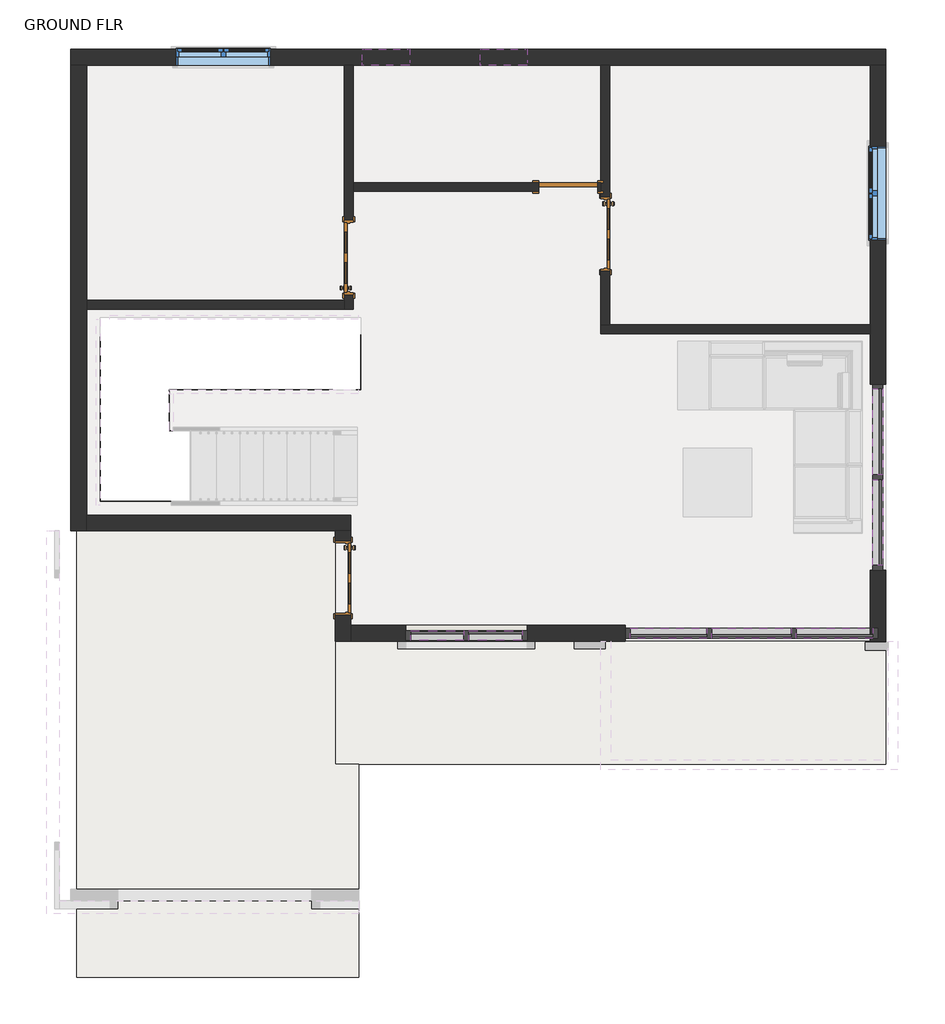
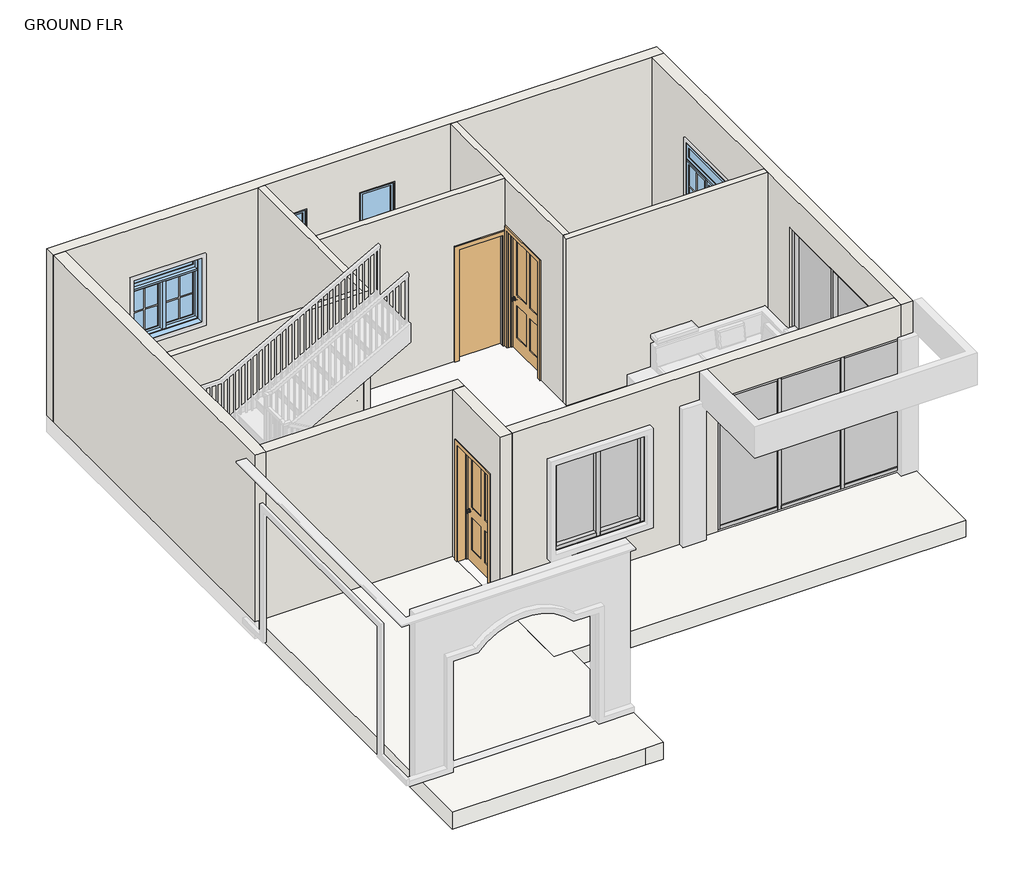
# One storey, part 1 of 3: 24 members, 11 walls, 7 plates, 7 slabs, 4 doors, 4 windows.
"""IFC4 building model written with IfcOpenShell, lengths in millimetres."""

from ifc_helpers import new_model, si_unit, frame, origin, origin_with_axes, place, context, project, spatial, polyline, outline, extrude, faceted_brep, transform, mapped, element, save
from components import door_2d5c49d3, door_c2926031, door_d8f5dbb5, member_5f1d7e17, member_aaf6ec4e, member_f0fea5a5, member_ee409385, member_a27facc5, member_7a2ba7d2, member_30308bf7, member_456a42a1, system_panel_glazed_72e6272a, system_panel_glazed_683b098e, system_panel_glazed_7ebbbc7e, system_panel_glazed_68324572, window_6846e476, window_ba962a69, window_3911def3

model = new_model("IFC4")

# Units and contexts
model_context = context("Model", 3, world=origin())
ifc_project = project(units=[si_unit("LENGTHUNIT", "METRE", prefix="MILLI")], contexts=[model_context])

# Site, building, storey
site = spatial("IfcSite", under=ifc_project)
building = spatial("IfcBuilding", under=site)
storey = spatial("IfcBuildingStorey", under=building, Name="GROUND FLR", Elevation=304.8)

# Doors
placement = place(None, origin())
door_shape = door_2d5c49d3(model_context)
element("IfcDoor", 1, ObjectType="Door-Interior-Single-4_Panel-Wood : 36\" x 84\"", at=placement, inside=storey, context=model_context, shape_type="MappedRepresentation", body=[
    mapped(door_shape, transform((-8111.9486584, -9455.4146616, 304.8), x_axis=(0.0, -1.0, 0.0), y_axis=(1.0, 0.0, 0.0), z_axis=(0.0, 0.0, 1.0))),
])
door_2_shape = door_c2926031(model_context)
element("IfcDoor", 2, ObjectType="Door-Interior-Single-4_Panel-Wood : 36\" x 84\"", at=placement, inside=storey, context=model_context, shape_type="MappedRepresentation", body=[
    mapped(door_2_shape, transform((-4711.4020642, -4994.5396616, 304.8), x_axis=(0.0, -1.0, 0.0), y_axis=(1.0, 0.0, 0.0), z_axis=(0.0, 0.0, 1.0))),
])
element("IfcDoor", 3, ObjectType="Door-Interior-Single-4_Panel-Wood : 36\" x 84\"", at=placement, inside=storey, context=model_context, shape_type="MappedRepresentation", body=[
    mapped(door_2_shape, transform((-8045.1520642, -5299.3396616, 304.8), x_axis=(0.0, 1.0, 0.0), y_axis=(-1.0, 0.0, 0.0), z_axis=(0.0, 0.0, 1.0))),
])
door_3_shape = door_d8f5dbb5(model_context)
element("IfcDoor", 4, ObjectType="Single-Flush : 30\" x 80\"", at=placement, inside=storey, context=model_context, shape_type="MappedRepresentation", body=[
    mapped(door_3_shape, transform((-5197.1770642, -4384.9396616, 304.8), x_axis=(1.0, 0.0, 0.0), y_axis=(0.0, 1.0, 0.0), z_axis=(0.0, 0.0, 1.0))),
])

# Members
member_shape = member_5f1d7e17(model_context)
element("IfcMember", 5, ObjectType="Rectangular Mullion : 2.5\" x 5\" rectangular", at=placement, inside=storey, context=model_context, shape_type="MappedRepresentation", body=[
    mapped(member_shape, transform((-5792.9495061, -10198.7950286, 2571.9634674), x_axis=(0.0, 0.0, 1.0), y_axis=(0.0, -1.0, 0.0), z_axis=(1.0, 0.0, 0.0))),
])
element("IfcMember", 6, ObjectType="Rectangular Mullion : 2.5\" x 5\" rectangular", at=placement, inside=storey, context=model_context, shape_type="MappedRepresentation", body=[
    mapped(member_shape, transform((-6548.5995061, -10198.7950286, 2571.9634674), x_axis=(0.0, 0.0, 1.0), y_axis=(0.0, -1.0, 0.0), z_axis=(1.0, 0.0, 0.0))),
])
element("IfcMember", 7, ObjectType="Rectangular Mullion : 2.5\" x 5\" rectangular", at=placement, inside=storey, context=model_context, shape_type="MappedRepresentation", body=[
    mapped(member_shape, transform((-7240.7495061, -10198.7950286, 947.4670086), x_axis=(0.0, 0.0, -1.0), y_axis=(0.0, -1.0, 0.0), z_axis=(-1.0, 0.0, 0.0))),
])
element("IfcMember", 8, ObjectType="Rectangular Mullion : 2.5\" x 5\" rectangular", at=placement, inside=storey, context=model_context, shape_type="MappedRepresentation", body=[
    mapped(member_shape, transform((-6485.0995061, -10198.7950286, 947.4670086), x_axis=(0.0, 0.0, -1.0), y_axis=(0.0, -1.0, 0.0), z_axis=(-1.0, 0.0, 0.0))),
])
member_2_shape = member_aaf6ec4e(model_context)
element("IfcMember", 9, ObjectType="Rectangular Mullion : 2.5\" x 5\" rectangular", at=placement, inside=storey, context=model_context, shape_type="MappedRepresentation", body=[
    mapped(member_2_shape, transform((-1180.9236584, -9288.7247117, 2743.2), x_axis=(0.0, 0.0, 1.0), y_axis=(-1.0, 0.0, 0.0), z_axis=(0.0, -1.0, 0.0))),
])
element("IfcMember", 10, ObjectType="Rectangular Mullion : 2.5\" x 5\" rectangular", at=placement, inside=storey, context=model_context, shape_type="MappedRepresentation", body=[
    mapped(member_2_shape, transform((-1180.9236584, -8113.9747117, 2743.2), x_axis=(0.0, 0.0, 1.0), y_axis=(-1.0, 0.0, 0.0), z_axis=(0.0, -1.0, 0.0))),
])
element("IfcMember", 11, ObjectType="Rectangular Mullion : 2.5\" x 5\" rectangular", at=placement, inside=storey, context=model_context, shape_type="MappedRepresentation", body=[
    mapped(member_2_shape, transform((-1180.9236584, -7002.7247117, 304.8), x_axis=(0.0, 0.0, -1.0), y_axis=(-1.0, 0.0, 0.0), z_axis=(0.0, 1.0, 0.0))),
])
element("IfcMember", 12, ObjectType="Rectangular Mullion : 2.5\" x 5\" rectangular", at=placement, inside=storey, context=model_context, shape_type="MappedRepresentation", body=[
    mapped(member_2_shape, transform((-1180.9236584, -8177.4747117, 304.8), x_axis=(0.0, 0.0, -1.0), y_axis=(-1.0, 0.0, 0.0), z_axis=(0.0, 1.0, 0.0))),
])
member_3_shape = member_f0fea5a5(model_context)
element("IfcMember", 13, ObjectType="Rectangular Mullion : 2.5\" x 5\" rectangular", at=placement, inside=storey, context=model_context, shape_type="MappedRepresentation", body=[
    mapped(member_3_shape, transform((-2273.1236585, -10169.7896616, 304.8), x_axis=(-1.0, 0.0, 0.0), y_axis=(0.0, 1.0, 0.0), z_axis=(0.0, 0.0, -1.0))),
])
element("IfcMember", 14, ObjectType="Rectangular Mullion : 2.5\" x 5\" rectangular", at=placement, inside=storey, context=model_context, shape_type="MappedRepresentation", body=[
    mapped(member_3_shape, transform((-3365.3236583, -10169.7896616, 304.8), x_axis=(-1.0, 0.0, 0.0), y_axis=(0.0, 1.0, 0.0), z_axis=(0.0, 0.0, -1.0))),
])
element("IfcMember", 15, ObjectType="Rectangular Mullion : 2.5\" x 5\" rectangular", at=placement, inside=storey, context=model_context, shape_type="MappedRepresentation", body=[
    mapped(member_3_shape, transform((-1180.9236584, -8145.7247117, 304.8), x_axis=(0.0, -1.0, 0.0), y_axis=(-1.0, 0.0, 0.0), z_axis=(0.0, 0.0, -1.0))),
])
member_4_shape = member_ee409385(model_context)
element("IfcMember", 16, ObjectType="Rectangular Mullion : 2.5\" x 5\" rectangular", at=placement, inside=storey, context=model_context, shape_type="MappedRepresentation", body=[
    mapped(member_4_shape, transform((-4457.5236584, -10169.7896616, 304.8), x_axis=(-1.0, 0.0, 0.0), y_axis=(0.0, 1.0, 0.0), z_axis=(0.0, 0.0, -1.0))),
])
element("IfcMember", 17, ObjectType="Rectangular Mullion : 2.5\" x 5\" rectangular", at=placement, inside=storey, context=model_context, shape_type="MappedRepresentation", body=[
    mapped(member_4_shape, transform((-1180.9236584, -9352.2247117, 304.8), x_axis=(0.0, -1.0, 0.0), y_axis=(-1.0, 0.0, 0.0), z_axis=(0.0, 0.0, -1.0))),
])
element("IfcMember", 18, ObjectType="Rectangular Mullion : 2.5\" x 5\" rectangular", at=placement, inside=storey, context=model_context, shape_type="MappedRepresentation", body=[
    mapped(member_4_shape, transform((-1180.9236584, -10169.7896616, 2743.2), x_axis=(1.0, 0.0, 0.0), y_axis=(0.0, 1.0, 0.0), z_axis=(0.0, 0.0, 1.0))),
])
element("IfcMember", 19, ObjectType="Rectangular Mullion : 2.5\" x 5\" rectangular", at=placement, inside=storey, context=model_context, shape_type="MappedRepresentation", body=[
    mapped(member_4_shape, transform((-1180.9236584, -6939.2247117, 2743.2), x_axis=(0.0, 1.0, 0.0), y_axis=(-1.0, 0.0, 0.0), z_axis=(0.0, 0.0, 1.0))),
])
member_5_shape = member_a27facc5(model_context)
element("IfcMember", 20, ObjectType="Rectangular Mullion : 2.5\" x 5\" rectangular", at=placement, inside=storey, context=model_context, shape_type="MappedRepresentation", body=[
    mapped(member_5_shape, transform((-6516.8495061, -10198.7950286, 947.4670086), x_axis=(1.0, 0.0, 0.0), y_axis=(0.0, -1.0, 0.0), z_axis=(0.0, 0.0, -1.0))),
])
member_6_shape = member_7a2ba7d2(model_context)
element("IfcMember", 21, ObjectType="Rectangular Mullion : 2.5\" x 5\" rectangular", at=placement, inside=storey, context=model_context, shape_type="MappedRepresentation", body=[
    mapped(member_6_shape, transform((-5729.4495061, -10198.7950286, 947.4670086), x_axis=(1.0, 0.0, 0.0), y_axis=(0.0, -1.0, 0.0), z_axis=(0.0, 0.0, -1.0))),
])
element("IfcMember", 22, ObjectType="Rectangular Mullion : 2.5\" x 5\" rectangular", at=placement, inside=storey, context=model_context, shape_type="MappedRepresentation", body=[
    mapped(member_6_shape, transform((-7304.2495061, -10198.7950286, 2571.9634674), x_axis=(-1.0, 0.0, 0.0), y_axis=(0.0, -1.0, 0.0), z_axis=(0.0, 0.0, 1.0))),
])
member_7_shape = member_30308bf7(model_context)
element("IfcMember", 23, ObjectType="Rectangular Mullion : 2.5\" x 5\" rectangular", at=placement, inside=storey, context=model_context, shape_type="MappedRepresentation", body=[
    mapped(member_7_shape, transform((-4394.0236584, -10169.7896616, 2743.2), x_axis=(0.0, 0.0, 1.0), y_axis=(0.0, 1.0, 0.0), z_axis=(-1.0, 0.0, 0.0))),
])
element("IfcMember", 24, ObjectType="Rectangular Mullion : 2.5\" x 5\" rectangular", at=placement, inside=storey, context=model_context, shape_type="MappedRepresentation", body=[
    mapped(member_7_shape, transform((-2241.3736585, -10169.7896616, 2743.2), x_axis=(0.0, 0.0, 1.0), y_axis=(0.0, 1.0, 0.0), z_axis=(-1.0, 0.0, 0.0))),
])
element("IfcMember", 25, ObjectType="Rectangular Mullion : 2.5\" x 5\" rectangular", at=placement, inside=storey, context=model_context, shape_type="MappedRepresentation", body=[
    mapped(member_7_shape, transform((-1244.4236584, -10169.7896616, 304.8), x_axis=(0.0, 0.0, -1.0), y_axis=(0.0, 1.0, 0.0), z_axis=(1.0, 0.0, 0.0))),
])
element("IfcMember", 26, ObjectType="Rectangular Mullion : 2.5\" x 5\" rectangular", at=placement, inside=storey, context=model_context, shape_type="MappedRepresentation", body=[
    mapped(member_7_shape, transform((-3397.0736583, -10169.7896616, 304.8), x_axis=(0.0, 0.0, -1.0), y_axis=(0.0, 1.0, 0.0), z_axis=(1.0, 0.0, 0.0))),
])
member_8_shape = member_456a42a1(model_context)
element("IfcMember", 27, ObjectType="Rectangular Mullion : 2.5\" x 5\" rectangular", at=placement, inside=storey, context=model_context, shape_type="MappedRepresentation", body=[
    mapped(member_8_shape, transform((-2304.8736585, -10169.7896616, 304.8), x_axis=(0.0, 0.0, -1.0), y_axis=(0.0, 1.0, 0.0), z_axis=(1.0, 0.0, 0.0))),
])
element("IfcMember", 28, ObjectType="Rectangular Mullion : 2.5\" x 5\" rectangular", at=placement, inside=storey, context=model_context, shape_type="MappedRepresentation", body=[
    mapped(member_8_shape, transform((-3333.5736583, -10169.7896616, 2743.2), x_axis=(0.0, 0.0, 1.0), y_axis=(0.0, 1.0, 0.0), z_axis=(-1.0, 0.0, 0.0))),
])

# Plates
system_panel_glazed_shape = system_panel_glazed_72e6272a(model_context)
element("IfcPlate", 29, ObjectType="System Panel : Glazed", at=placement, inside=storey, context=model_context, shape_type="MappedRepresentation", body=[
    mapped(system_panel_glazed_shape, transform((-1180.9236584, -7558.3497117, 368.3), x_axis=(0.0, -1.0, 0.0), y_axis=(1.0, 0.0, 0.0), z_axis=(0.0, 0.0, 1.0))),
])
element("IfcPlate", 30, ObjectType="System Panel : Glazed", at=placement, inside=storey, context=model_context, shape_type="MappedRepresentation", body=[
    mapped(system_panel_glazed_shape, transform((-1180.9236584, -8733.0997117, 368.3), x_axis=(0.0, -1.0, 0.0), y_axis=(1.0, 0.0, 0.0), z_axis=(0.0, 0.0, 1.0))),
])
system_panel_glazed_2_shape = system_panel_glazed_683b098e(model_context)
element("IfcPlate", 31, ObjectType="System Panel : Glazed", at=placement, inside=storey, context=model_context, shape_type="MappedRepresentation", body=[
    mapped(system_panel_glazed_2_shape, transform((-6894.6745061, -10198.7950286, 1010.9670086), x_axis=(1.0, 0.0, 0.0), y_axis=(0.0, 1.0, 0.0), z_axis=(0.0, 0.0, 1.0))),
])
element("IfcPlate", 32, ObjectType="System Panel : Glazed", at=placement, inside=storey, context=model_context, shape_type="MappedRepresentation", body=[
    mapped(system_panel_glazed_2_shape, transform((-6139.0245061, -10198.7950286, 1010.9670086), x_axis=(1.0, 0.0, 0.0), y_axis=(0.0, 1.0, 0.0), z_axis=(0.0, 0.0, 1.0))),
])
system_panel_glazed_3_shape = system_panel_glazed_7ebbbc7e(model_context)
element("IfcPlate", 33, ObjectType="System Panel : Glazed", at=placement, inside=storey, context=model_context, shape_type="MappedRepresentation", body=[
    mapped(system_panel_glazed_3_shape, transform((-1742.8986584, -10169.7896616, 368.3), x_axis=(-1.0, 0.0, 0.0), y_axis=(0.0, -1.0, 0.0), z_axis=(0.0, 0.0, 1.0))),
])
element("IfcPlate", 34, ObjectType="System Panel : Glazed", at=placement, inside=storey, context=model_context, shape_type="MappedRepresentation", body=[
    mapped(system_panel_glazed_3_shape, transform((-3895.5486583, -10169.7896616, 368.3), x_axis=(-1.0, 0.0, 0.0), y_axis=(0.0, -1.0, 0.0), z_axis=(0.0, 0.0, 1.0))),
])
system_panel_glazed_4_shape = system_panel_glazed_68324572(model_context)
element("IfcPlate", 35, ObjectType="System Panel : Glazed", at=placement, inside=storey, context=model_context, shape_type="MappedRepresentation", body=[
    mapped(system_panel_glazed_4_shape, transform((-2819.2236584, -10169.7896616, 368.3), x_axis=(-1.0, 0.0, 0.0), y_axis=(0.0, -1.0, 0.0), z_axis=(0.0, 0.0, 1.0))),
])

# Slabs
element("IfcSlab", 36, ObjectType="FLOORING 1'", at=placement, inside=storey, context=model_context, shape_type="SweptSolid", body=[
    extrude(outline(polyline([(-8216.7236584, -10271.3896616), (-1079.3236584, -10271.3896616), (-1079.3236584, -11867.7407184), (-8216.7236584, -11867.7407184), (-8216.7236584, -10271.3896616)])), origin_with_axes(), (0.0, 0.0, 1.0), 304.8),
])
element("IfcSlab", 37, ObjectType="FLOORING 1'", at=placement, inside=storey, context=model_context, shape_type="SweptSolid", body=[
    extrude(outline(polyline([(-11569.5236584, -8842.6396616), (-8216.7236584, -8842.6396616), (-8216.7236584, -11867.7407184), (-7911.9236584, -11867.7407184), (-7911.9236584, -14633.8396616), (-8216.7236584, -14633.8396616), (-11569.5236584, -14633.8396616), (-11569.5236584, -8842.6396616)])), origin_with_axes(), (0.0, 0.0, 1.0), 304.8),
])
element("IfcSlab", 38, ObjectType="Generic - 12\"", at=placement, inside=storey, context=model_context, shape_type="Brep", body=[
    faceted_brep([(-8251.5270642, -2868.8747117, -304.8), (-8251.5270642, -6018.4747117, -304.8), (-11339.0293601, -6018.4747117, -304.8), (-11339.0293601, -2868.8747117, -304.8), (-8251.5270642, -2868.8747117, 0.0), (-11339.0293601, -2868.8747117, 0.0), (-11339.0293601, -6018.4747117, 0.0), (-8251.5270642, -6018.4747117, 0.0), (-8251.5270642, -5993.0747117, 0.0)], [[[0, 1, 2, 3]], [[4, 5, 6, 7, 8]], [[1, 0, 4, 8, 7]], [[2, 1, 7, 6]], [[3, 2, 6, 5]], [[0, 3, 5, 4]]]),
])
element("IfcSlab", 39, ObjectType="Generic - 12\"", at=placement, inside=storey, context=model_context, shape_type="SweptSolid", body=[
    extrude(outline(polyline([(-1351.9658472, -6297.8747117), (-1351.9658472, -9984.0050402), (-4492.3270642, -9984.0050402), (-4492.3270642, -6297.8747117), (-1351.9658472, -6297.8747117)])), frame((0.0, 0.0, -304.8), z_axis=(0.0, 0.0, 1.0), x_axis=(1.0, 0.0, 0.0)), (0.0, 0.0, 1.0), 304.8),
])
element("IfcSlab", 40, ObjectType="Generic - 12\"", at=placement, inside=storey, context=model_context, shape_type="SweptSolid", body=[
    extrude(outline(polyline([(-4801.7464557, -6297.8747117), (-4801.7464557, -9984.0050402), (-7942.1076727, -9984.0050402), (-7942.1076727, -8461.6396616), (-7930.9736584, -8461.6396616), (-7930.9736584, -7547.2396616), (-7942.1076727, -7547.2396616), (-7942.1076727, -7013.8396616), (-7889.5770642, -7013.8396616), (-7889.5770642, -6297.8747117), (-4801.7464557, -6297.8747117)])), frame((0.0, 0.0, -304.8), z_axis=(0.0, 0.0, 1.0), x_axis=(1.0, 0.0, 0.0)), (0.0, 0.0, 1.0), 304.8),
])
element("IfcSlab", 41, ObjectType="Generic - 12\"", at=placement, inside=storey, context=model_context, shape_type="SweptSolid", body=[
    extrude(outline(polyline([(-8251.6377222, -8597.9373391), (-11339.0293601, -8597.9373391), (-11339.0293601, -6323.2747117), (-11264.7236584, -6323.2747117), (-11264.7236584, -8461.6396616), (-8251.6377222, -8461.6396616), (-8251.6377222, -8597.9373391)])), frame((0.0, 0.0, -304.8), z_axis=(0.0, 0.0, 1.0), x_axis=(1.0, 0.0, 0.0)), (0.0, 0.0, 1.0), 304.8),
    extrude(outline(polyline([(-8251.6377222, -7013.8396616), (-8251.6377222, -7547.2396616), (-10369.3736584, -7547.2396616), (-10369.3736584, -7013.8396616), (-8251.6377222, -7013.8396616)])), frame((0.0, 0.0, -304.8), z_axis=(0.0, 0.0, 1.0), x_axis=(1.0, 0.0, 0.0)), (0.0, 0.0, 1.0), 304.8),
])
element("IfcSlab", 42, ObjectType="Generic - 12\"", at=placement, inside=storey, context=model_context, shape_type="Brep", body=[
    faceted_brep([(-8226.1270642, -8902.7191027, -304.8), (-8226.1270642, -9984.0050402, -304.8), (-8226.1270642, -10288.8050402, -304.8), (-8226.1270642, -13183.002305, -304.8), (-11339.0293601, -13183.002305, -304.8), (-11339.0293601, -8902.7191027, -304.8), (-8226.1270642, -8902.7191027, 0.0), (-8251.5270642, -8902.7191027, 0.0), (-11339.0293601, -8902.7191027, 0.0), (-11339.0293601, -13183.002305, 0.0), (-8226.1270642, -13183.002305, 0.0), (-8226.1270642, -10288.8050402, 0.0), (-8226.1270642, -9984.0050402, 0.0)], [[[0, 1, 2, 3, 4, 5]], [[6, 7, 8, 9, 10, 11, 12]], [[3, 2, 1, 0, 6, 12, 11, 10]], [[4, 3, 10, 9]], [[5, 4, 9, 8]], [[0, 5, 8, 7, 6]]]),
])

# Walls
element("IfcWall", 43, ObjectType="EXTERIOR 8'", at=placement, inside=storey, context=model_context, shape_type="Brep", body=[
    faceted_brep([(-11645.7236584, -2803.7896616, 304.8), (-11442.5236584, -2803.7896616, 304.8), (-8099.1270642, -2803.7896616, 304.8), (-7984.8270642, -2803.7896616, 304.8), (-4771.7270642, -2803.7896616, 304.8), (-4657.4270642, -2803.7896616, 304.8), (-1282.5236584, -2803.7896616, 304.8), (-1079.3236584, -2803.7896616, 304.8), (-1079.3236584, -2803.7896616, 3352.8), (-1282.5236584, -2803.7896616, 3352.8), (-4657.4270642, -2803.7896616, 3352.8), (-4771.7270642, -2803.7896616, 3352.8), (-7984.8270642, -2803.7896616, 3352.8), (-8099.1270642, -2803.7896616, 3352.8), (-11442.5236584, -2803.7896616, 3352.8), (-11645.7236584, -2803.7896616, 3352.8), (-9057.9770642, -2803.7896616, 2438.4), (-9057.9770642, -2803.7896616, 1219.2), (-10277.1770642, -2803.7896616, 1219.2), (-10277.1770642, -2803.7896616, 2438.4), (-6340.1770642, -2803.7896616, 2641.6), (-5730.5770642, -2803.7896616, 2641.6), (-5730.5770642, -2803.7896616, 2032.0), (-6340.1770642, -2803.7896616, 2032.0), (-7864.1770642, -2803.7896616, 2667.0), (-7254.5770642, -2803.7896616, 2667.0), (-7254.5770642, -2803.7896616, 2057.4), (-7864.1770642, -2803.7896616, 2057.4), (-11645.7236584, -2600.5896616, 304.8), (-11645.7236584, -2600.5896616, 3352.8), (-1079.3236584, -2600.5896616, 3352.8), (-1079.3236584, -2600.5896616, 304.8), (-9057.9770642, -2600.5896616, 2438.4), (-10277.1770642, -2600.5896616, 2438.4), (-10277.1770642, -2600.5896616, 1219.2), (-9057.9770642, -2600.5896616, 1219.2), (-6340.1770642, -2600.5896616, 2641.6), (-6340.1770642, -2600.5896616, 2032.0), (-5730.5770642, -2600.5896616, 2032.0), (-5730.5770642, -2600.5896616, 2641.6), (-7864.1770642, -2600.5896616, 2667.0), (-7864.1770642, -2600.5896616, 2057.4), (-7254.5770642, -2600.5896616, 2057.4), (-7254.5770642, -2600.5896616, 2667.0)], [[[0, 1, 2, 3, 4, 5, 6, 7, 8, 9, 10, 11, 12, 13, 14, 15], [16, 17, 18, 19], [20, 21, 22, 23], [24, 25, 26, 27]], [[28, 29, 30, 31], [32, 33, 34, 35], [36, 37, 38, 39], [40, 41, 42, 43]], [[7, 6, 5, 4, 3, 2, 1, 0, 28, 31]], [[15, 14, 13, 12, 11, 10, 9, 8, 30, 29]], [[8, 7, 31, 30]], [[0, 15, 29, 28]], [[17, 16, 32, 35]], [[18, 17, 35, 34]], [[19, 18, 34, 33]], [[16, 19, 33, 32]], [[37, 36, 20, 23]], [[38, 37, 23, 22]], [[39, 38, 22, 21]], [[36, 39, 21, 20]], [[41, 40, 24, 27]], [[42, 41, 27, 26]], [[43, 42, 26, 25]], [[40, 43, 25, 24]]]),
])
element("IfcWall", 44, ObjectType="EXTERIOR 8'", at=placement, inside=storey, context=model_context, shape_type="Brep", body=[
    faceted_brep([(-1282.5236584, -10271.3896616, 3352.8), (-1282.5236584, -10068.1896616, 3352.8), (-1282.5236584, -6285.1747117, 3352.8), (-1282.5236584, -6170.8747117, 3352.8), (-1282.5236584, -2803.7896616, 3352.8), (-1282.5236584, -2803.7896616, 304.8), (-1282.5236584, -6170.8747117, 304.8), (-1282.5236584, -6285.1747117, 304.8), (-1282.5236584, -6939.2247117, 304.8), (-1282.5236584, -6939.2247117, 2743.2), (-1282.5236584, -9352.2247117, 2743.2), (-1282.5236584, -9352.2247117, 304.8), (-1282.5236584, -10271.3896616, 304.8), (-1282.5236584, -10271.3896616, 2743.2), (-1282.5236584, -5074.7071866, 2438.4), (-1282.5236584, -5074.7071866, 1219.2), (-1282.5236584, -3855.5071866, 1219.2), (-1282.5236584, -3855.5071866, 2438.4), (-1079.3236584, -2803.7896616, 3352.8), (-1079.3236584, -10271.3896616, 3352.8), (-1079.3236584, -10271.3896616, 304.8), (-1079.3236584, -9352.2247117, 304.8), (-1079.3236584, -9352.2247117, 2743.2), (-1079.3236584, -6939.2247117, 2743.2), (-1079.3236584, -6939.2247117, 304.8), (-1079.3236584, -2803.7896616, 304.8), (-1079.3236584, -5074.7071866, 2438.4), (-1079.3236584, -3855.5071866, 2438.4), (-1079.3236584, -3855.5071866, 1219.2), (-1079.3236584, -5074.7071866, 1219.2)], [[[0, 1, 2, 3, 4, 5, 6, 7, 8, 9, 10, 11, 12, 13], [14, 15, 16, 17]], [[18, 19, 20, 21, 22, 23, 24, 25], [26, 27, 28, 29]], [[5, 25, 24, 8, 7, 6]], [[20, 12, 11, 21]], [[4, 3, 2, 1, 0, 19, 18]], [[5, 4, 18, 25]], [[0, 13, 12, 20, 19]], [[15, 14, 26, 29]], [[16, 15, 29, 28]], [[17, 16, 28, 27]], [[14, 17, 27, 26]], [[23, 9, 8, 24]], [[9, 23, 22, 10]], [[10, 22, 21, 11]]]),
])
element("IfcWall", 45, ObjectType="EXTERIOR 8'", at=placement, inside=storey, context=model_context, shape_type="Brep", body=[
    faceted_brep([(-11645.7236584, -2803.7896616, 304.8), (-11645.7236584, -8842.6396616, 304.8), (-11645.7236584, -8842.6396616, 3352.8), (-11645.7236584, -2803.7896616, 3352.8), (-11442.5236584, -2803.7896616, 304.8), (-11442.5236584, -2803.7896616, 3352.8), (-11442.5236584, -5851.7896616, 3352.8), (-11442.5236584, -5966.0896616, 3352.8), (-11442.5236584, -8639.4396616, 3352.8), (-11442.5236584, -8842.6396616, 3352.8), (-11442.5236584, -8842.6396616, 304.8), (-11442.5236584, -8639.4396616, 304.8), (-11442.5236584, -5966.0896616, 304.8), (-11442.5236584, -5851.7896616, 304.8)], [[[0, 1, 2, 3]], [[4, 5, 6, 7, 8, 9, 10, 11, 12, 13]], [[1, 0, 4, 13, 12, 11, 10]], [[3, 2, 9, 8, 7, 6, 5]], [[0, 3, 5, 4]], [[2, 1, 10, 9]]]),
])
element("IfcWall", 46, ObjectType="EXTERIOR 8'", at=placement, inside=storey, context=model_context, shape_type="Brep", body=[
    faceted_brep([(-11442.5236584, -8842.6396616, 304.8), (-8216.7236584, -8842.6396616, 304.8), (-8013.5236584, -8842.6396616, 304.8), (-8013.5236584, -8842.6396616, 3352.8), (-8216.7236584, -8842.6396616, 3352.8), (-11442.5236584, -8842.6396616, 3352.8), (-11442.5236584, -8639.4396616, 304.8), (-11442.5236584, -8639.4396616, 3352.8), (-8013.5236584, -8639.4396616, 3352.8), (-8013.5236584, -8639.4396616, 304.8)], [[[0, 1, 2, 3, 4, 5]], [[6, 7, 8, 9]], [[2, 1, 0, 6, 9]], [[5, 4, 3, 8, 7]], [[0, 5, 7, 6]], [[3, 2, 9, 8]]]),
])
element("IfcWall", 47, ObjectType="EXTERIOR 8'", at=placement, inside=storey, context=model_context, shape_type="Brep", body=[
    faceted_brep([(-8216.7236584, -10271.3896616, 3352.8), (-8216.7236584, -8842.6396616, 3352.8), (-8216.7236584, -8842.6396616, 304.8), (-8216.7236584, -8972.8146616, 304.8), (-8216.7236584, -8972.8146616, 2463.8), (-8216.7236584, -9938.0146616, 2463.8), (-8216.7236584, -9938.0146616, 304.8), (-8216.7236584, -10271.3896616, 304.8), (-8013.5236584, -8842.6396616, 3352.8), (-8013.5236584, -10068.1896616, 3352.8), (-8013.5236584, -10271.3896616, 3352.8), (-8013.5236584, -10271.3896616, 304.8), (-8013.5236584, -10068.1896616, 304.8), (-8013.5236584, -9938.0146616, 304.8), (-8013.5236584, -9938.0146616, 2463.8), (-8013.5236584, -8972.8146616, 2463.8), (-8013.5236584, -8972.8146616, 304.8), (-8013.5236584, -8842.6396616, 304.8)], [[[0, 1, 2, 3, 4, 5, 6, 7]], [[8, 9, 10, 11, 12, 13, 14, 15, 16, 17]], [[2, 17, 16, 3]], [[11, 7, 6, 13, 12]], [[1, 0, 10, 9, 8]], [[2, 1, 8, 17]], [[0, 7, 11, 10]], [[5, 14, 13, 6]], [[14, 5, 4, 15]], [[15, 4, 3, 16]]]),
])
element("IfcWall", 48, ObjectType="EXTERIOR 8'", at=placement, inside=storey, context=model_context, shape_type="SweptSolid", body=[
    extrude(outline(polyline([(3352.8, -1282.5236584), (3352.8, -8013.5236584), (304.8, -8013.5236584), (304.8, -4457.5236584), (2743.2, -4457.5236584), (2743.2, -1282.5236584), (3352.8, -1282.5236584)]), holes=[polyline([(947.4670086, -7304.2495061), (2571.9634674, -7304.2495061), (2571.9634674, -5729.4495061), (947.4670086, -5729.4495061), (947.4670086, -7304.2495061)])]), frame((0.0, -10271.3896616, 0.0), z_axis=(0.0, 1.0, 0.0), x_axis=(0.0, 0.0, 1.0)), (0.0, 0.0, 1.0), 203.2),
])
element("IfcWall", 49, ObjectType="interior wall 4.5\"", at=placement, inside=storey, context=model_context, shape_type="Brep", body=[
    faceted_brep([(-1282.5236584, -6170.8747117, 304.8), (-4657.4270642, -6170.8747117, 304.8), (-4771.7270642, -6170.8747117, 304.8), (-4771.7270642, -6170.8747117, 3352.8), (-4657.4270642, -6170.8747117, 3352.8), (-1282.5236584, -6170.8747117, 3352.8), (-1282.5236584, -6285.1747117, 304.8), (-1282.5236584, -6285.1747117, 3352.8), (-4771.7270642, -6285.1747117, 3352.8), (-4771.7270642, -6285.1747117, 304.8)], [[[0, 1, 2, 3, 4, 5]], [[6, 7, 8, 9]], [[2, 1, 0, 6, 9]], [[5, 4, 3, 8, 7]], [[0, 5, 7, 6]], [[3, 2, 9, 8]]]),
])
element("IfcWall", 50, ObjectType="interior wall 4.5\"", at=placement, inside=storey, context=model_context, shape_type="Brep", body=[
    faceted_brep([(-4771.7270642, -6170.8747117, 3352.8), (-4771.7270642, -4442.0896616, 3352.8), (-4771.7270642, -4327.7896616, 3352.8), (-4771.7270642, -2803.7896616, 3352.8), (-4771.7270642, -2803.7896616, 304.8), (-4771.7270642, -4327.7896616, 304.8), (-4771.7270642, -4442.0896616, 304.8), (-4771.7270642, -4511.9396616, 304.8), (-4771.7270642, -4511.9396616, 2463.8), (-4771.7270642, -5477.1396616, 2463.8), (-4771.7270642, -5477.1396616, 304.8), (-4771.7270642, -6170.8747117, 304.8), (-4657.4270642, -2803.7896616, 3352.8), (-4657.4270642, -6170.8747117, 3352.8), (-4657.4270642, -6170.8747117, 304.8), (-4657.4270642, -5477.1396616, 304.8), (-4657.4270642, -5477.1396616, 2463.8), (-4657.4270642, -4511.9396616, 2463.8), (-4657.4270642, -4511.9396616, 304.8), (-4657.4270642, -2803.7896616, 304.8)], [[[0, 1, 2, 3, 4, 5, 6, 7, 8, 9, 10, 11]], [[12, 13, 14, 15, 16, 17, 18, 19]], [[4, 19, 18, 7, 6, 5]], [[14, 11, 10, 15]], [[3, 2, 1, 0, 13, 12]], [[4, 3, 12, 19]], [[0, 11, 14, 13]], [[9, 16, 15, 10]], [[16, 9, 8, 17]], [[17, 8, 7, 18]]]),
])
element("IfcWall", 51, ObjectType="interior wall 4.5\"", at=placement, inside=storey, context=model_context, shape_type="Brep", body=[
    faceted_brep([(-8099.1270642, -5966.0896616, 3352.8), (-8099.1270642, -5851.7896616, 3352.8), (-8099.1270642, -2803.7896616, 3352.8), (-8099.1270642, -2803.7896616, 304.8), (-8099.1270642, -4816.7396616, 304.8), (-8099.1270642, -4816.7396616, 2463.8), (-8099.1270642, -5781.9396616, 2463.8), (-8099.1270642, -5781.9396616, 304.8), (-8099.1270642, -5851.7896616, 304.8), (-8099.1270642, -5966.0896616, 304.8), (-7984.8270642, -2803.7896616, 3352.8), (-7984.8270642, -4327.7896616, 3352.8), (-7984.8270642, -4442.0896616, 3352.8), (-7984.8270642, -5966.0896616, 3352.8), (-7984.8270642, -5966.0896616, 304.8), (-7984.8270642, -5781.9396616, 304.8), (-7984.8270642, -5781.9396616, 2463.8), (-7984.8270642, -4816.7396616, 2463.8), (-7984.8270642, -4816.7396616, 304.8), (-7984.8270642, -4442.0896616, 304.8), (-7984.8270642, -4327.7896616, 304.8), (-7984.8270642, -2803.7896616, 304.8)], [[[0, 1, 2, 3, 4, 5, 6, 7, 8, 9]], [[10, 11, 12, 13, 14, 15, 16, 17, 18, 19, 20, 21]], [[3, 21, 20, 19, 18, 4]], [[14, 9, 8, 7, 15]], [[2, 1, 0, 13, 12, 11, 10]], [[3, 2, 10, 21]], [[0, 9, 14, 13]], [[17, 5, 4, 18]], [[5, 17, 16, 6]], [[6, 16, 15, 7]]]),
])
element("IfcWall", 52, ObjectType="interior wall 4.5\"", at=placement, inside=storey, context=model_context, shape_type="SweptSolid", body=[
    extrude(outline(polyline([(-11442.5236584, -5851.7896616), (-8099.1270642, -5851.7896616), (-8099.1270642, -5966.0896616), (-11442.5236584, -5966.0896616), (-11442.5236584, -5851.7896616)])), frame((0.0, 0.0, 304.8), z_axis=(0.0, 0.0, 1.0), x_axis=(1.0, 0.0, 0.0)), (0.0, 0.0, 1.0), 3048.0),
])
element("IfcWall", 53, ObjectType="interior wall 4.5\"", at=placement, inside=storey, context=model_context, shape_type="SweptSolid", body=[
    extrude(outline(polyline([(2336.8, -4816.1770642), (304.8, -4816.1770642), (304.8, -4771.7270642), (3352.8, -4771.7270642), (3352.8, -7984.8270642), (304.8, -7984.8270642), (304.8, -5578.1770642), (2336.8, -5578.1770642), (2336.8, -4816.1770642)])), frame((0.0, -4442.0896616, 0.0), z_axis=(0.0, 1.0, 0.0), x_axis=(0.0, 0.0, 1.0)), (0.0, 0.0, 1.0), 114.3),
])

# Windows
window_shape = window_6846e476(model_context)
element("IfcWindow", 54, ObjectType="Fixed : 24\" x 24\"", at=placement, inside=storey, context=model_context, shape_type="MappedRepresentation", body=[
    mapped(window_shape, transform((-6073.4770642, -2702.1896616, 1117.6), x_axis=(-1.0, 0.0, 0.0), y_axis=(0.0, -1.0, 0.0), z_axis=(0.0, 0.0, 1.0))),
])
element("IfcWindow", 55, ObjectType="Fixed : 24\" x 24\"", at=placement, inside=storey, context=model_context, shape_type="MappedRepresentation", body=[
    mapped(window_shape, transform((-7597.4770642, -2702.1896616, 1143.0), x_axis=(-1.0, 0.0, 0.0), y_axis=(0.0, -1.0, 0.0), z_axis=(0.0, 0.0, 1.0))),
])
window_2_shape = window_ba962a69(model_context)
element("IfcWindow", 56, ObjectType="Window-Casement-Double-Transom : 48\" x 48\"", at=placement, inside=storey, context=model_context, shape_type="MappedRepresentation", body=[
    mapped(window_2_shape, transform((-9667.5770642, -2702.1896616, 304.8), x_axis=(1.0, 0.0, 0.0), y_axis=(0.0, 1.0, 0.0), z_axis=(0.0, 0.0, 1.0))),
])
window_3_shape = window_3911def3(model_context)
element("IfcWindow", 57, ObjectType="Window-Casement-Double-Transom : 48\" x 48\"", at=placement, inside=storey, context=model_context, shape_type="MappedRepresentation", body=[
    mapped(window_3_shape, transform((-1180.9236584, -4465.1071866, 304.8), x_axis=(0.0, -1.0, 0.0), y_axis=(1.0, 0.0, 0.0), z_axis=(0.0, 0.0, 1.0))),
])

save(model, "model.ifc")

# Revit data of these elements
# Type "Door-Interior-Single-4_Panel-Wood : 36\" x 84\""
#   Type Mark = "8"
#   Assembly Code = "C1020300"
#   Analytic Construction = "Wooden"
#   Top Rail = 0' - 4 11/16"
#   Thickness = 0' - 1 3/8"
#   Thermal Resistance (R) = 2.5876 (h·ft²·°F)/BTU
#   Swing Angle [instance default] = 90.00°
#   Stiles = 0' - 4 3/4"
#   Rough Width = 3' - 2"
#   Rough Height = 7' - 1"
#   Mullion = 0' - 4 1/2"
#   Lock Rail = 0' - 7 1/2"
#   Height = 7' - 0"
#   Width = 3' - 0"
#   Heat Transfer Coefficient (U) = 0.3865 BTU/(h·ft²·°F)
#   Bottom Rail = 0' - 9 1/8"
#   Trim Material = Cherry
#   Panel Material = Cherry
#   Frame Material = Cherry
#   Door Handle Material = Aluminum
#   Visual Light Transmittance = 0
#   Solar Heat Gain Coefficient = 0
#   Wall Closure = (empty or 0)
#   Function = (empty or 0)
# Type "Single-Flush : 30\" x 80\""
#   Type Mark = "5"
#   Construction Type Id = "MDOOR"
#   Assembly Code = "C1020"
#   Analytic Construction = "Metal"
#   Thickness = 0' - 2"
#   Heat Transfer Coefficient (U) = 0.651978 BTU/(h·ft²·°F)
#   Height = 6' - 8"
#   Trim Projection Ext = 0' - 1"
#   Trim Projection Int = 0' - 1"
#   Trim Width = 0' - 3"
#   Width = 2' - 6"
#   Define Thermal Properties by = 1
#   Define Thermal Properties by = 1
#   Door Material = Door - Panel
#   Frame Material = Door - Frame
#   Visual Light Transmittance = 0
#   Solar Heat Gain Coefficient = 0
#   Function = (empty or 0)
#   Wall Closure = (empty or 0)
# Type "Rectangular Mullion : 2.5\" x 5\" rectangular"
#   built-in parameter 1007304 = 0.416667 (stored number, unit not read)
#   built-in parameter 1007301 = 0.104167 (stored number, unit not read)
#   built-in parameter 1007300 = 0.104167 (stored number, unit not read)
# Type "System Panel : Glazed"
#   Construction Type Id = "GSP4R"
#   Analytic Construction = "1/8 in Pilkington single glazing"
#   Visual Light Transmittance = 0.9
#   Solar Heat Gain Coefficient = 0.86
#   Heat Transfer Coefficient (U) = 1.18115 BTU/(h·ft²·°F)
#   Define Thermal Properties by = 1
# Type "FLOORING 1'"
#   Assembly Code = "B1010"
#   Function = 0
#   Layers, outside or top first: 1' - 0" "MARBLE FLOORING 6\"" (function 1)
# Type "Generic - 12\""
#   Assembly Code = "B1010"
#   Function = 0
#   Layers, outside or top first: 1' - 0" no material (function 1)
# Type "EXTERIOR 8'"
#   Assembly Code = "B2010"
#   Layers, outside or top first: 0' - 8" "beige colour" (function 1)
# Type "interior wall 4.5\""
#   Assembly Code = "B2010"
#   Layers, outside or top first: 0' - 4 1/2" "beige colour" (function 1)
# Type "Fixed : 24\" x 24\""
#   Type Mark = "3"
#   Construction Type Id = "GSP4R"
#   Assembly Code = "B2020100"
#   Analytic Construction = "1/8 in Pilkington single glazing"
#   Visual Light Transmittance = 0.9
#   Solar Heat Gain Coefficient = 0.78
#   Heat Transfer Coefficient (U) = 0.6496 BTU/(h·ft²·°F)
#   Height = 2' - 0"
#   Default Sill Height = 3' - 0"
#   Width = 2' - 0"
#   Window Inset = 0' - 0 3/4"
#   Define Thermal Properties by = 1
#   Define Thermal Properties by = 1
#   Glass Pane Material = Glass
#   Sash Material = Sash
#   Wall Closure = (empty or 0)
# Type "Window-Casement-Double-Transom : 48\" x 48\""
#   Type Mark = "18"
#   Fire Rating = "0.5h"
#   Assembly Code = "B2020100"
#   Analytic Construction = "Double glazing - domestic"
#   Window Inset [instance default] = 0' - 0"
#   Wall Thickness [instance default] = 0' - 6"
#   Interior Wall Closure [instance default] = 0' - 2 1/4"
#   Half Width = 2' - 0"
#   Visual Light Transmittance = 0.81
#   Transom Height = 1' - 0"
#   Thermal Resistance (R) = 1.8146 (h·ft²·°F)/BTU
#   Solar Heat Gain Coefficient = 0.76
#   Rough Width = 4' - 0 1/2"
#   Rough Height = 4' - 0 1/2"
#   Open Window Height = 3' - 0"
#   Height = 4' - 0"
#   Heat Transfer Coefficient (U) = 0.5511 BTU/(h·ft²·°F)
#   Frame Extension [instance default] = 0' - 0 1/4"
#   Exterior Wall Closure [instance default] = 0' - 1 1/4"
#   Extension Jamb [instance default] = 0' - 2 1/4"
#   Default Sill Height = 3' - 0"
#   Width = 4' - 0"
#   Muntin Visibility = yes
#   Interior Trim Visibility [instance default] = yes
#   Exterior Trim Visibility [instance default] = yes
#   Extension Jamb Visibility [instance default] = yes
#   Interior Trim Material = Wood - Stained
#   Muntin Pattern = Muntin Pattern_2x2 : Muntin Pattern_2x2
#   Interior Trim = Trim-Window-Interior-Flat : Picture Frame
#   Interior Frame Material = Wood - Stained
#   Glass Panel Material = Glass
#   Exterior Trim Material = Clad - White
#   Exterior Trim = Trim-Window-Exterior-Flat : with Sill
#   Exterior Frame Material = Clad - White
#   Wall Closure = (empty or 0)
# Elements 1, 2, 3 (IfcDoor, "Door-Interior-Single-4_Panel-Wood : 36\" x 84\"")
#   Swing Angle = 90.00°
#   Phase Created = New Construction
#   Materials on its faces: "Cherry", "Aluminum"
# Element 4 (IfcDoor, "Single-Flush : 30\" x 80\"")
#   Phase Created = New Construction
#   Materials on its faces: "Door - Frame", "Door - Panel"
# Elements 5, 6, 7, 8, 9, 10, 11, 12, 13, 14, 15, 16, 17, 18, 19, 20, 21, 22, 23, 24, 25, 26, 27, 28 (IfcMember, "Rectangular Mullion : 2.5\" x 5\" rectangular")
#   Phase Created = New Construction
#   Materials on its faces: "Aluminum"
# Elements 29, 30, 31, 32, 33, 34, 35 (IfcPlate, "System Panel : Glazed")
#   Phase Created = New Construction
#   Materials on its faces: "Glass"
# Elements 36, 37 (IfcSlab, "FLOORING 1'")
#   built-in parameter 1001955 = 3.14159 (stored number, unit not read)
#   Height Offset From Level = 0' - 0"
#   Phase Created = New Construction
#   Materials on its faces: "MARBLE FLOORING 6\""
# Elements 38, 39, 40, 41, 42 (IfcSlab, "Generic - 12\"")
#   Height Offset From Level = -1' - 0"
#   built-in parameter 1001954 = 1
#   Phase Created = New Construction
#   Materials on its faces: "Default Floor"
# Elements 43, 44, 45, 46, 47, 48 (IfcWall, "EXTERIOR 8'")
#   Top Offset = 0' - 0"
#   Base Offset = 0' - 0"
#   wall height = 10' - 0"
#   Phase Created = New Construction
#   Base Constraint = GROUND FLR
#   Top Constraint = FIRST FLR
#   Materials on its faces: "beige colour"
# Elements 49, 50, 51, 52, 53 (IfcWall, "interior wall 4.5\"")
#   Top Offset = 0' - 0"
#   Base Offset = 0' - 0"
#   wall height = 10' - 0"
#   Phase Created = New Construction
#   Base Constraint = GROUND FLR
#   Top Constraint = FIRST FLR
#   Materials on its faces: "beige colour"
# Element 54 (IfcWindow, "Fixed : 24\" x 24\"")
#   Mark = "3"
#   Phase Created = New Construction
#   Materials on its faces: "Sash", "Glass"
# Element 55 (IfcWindow, "Fixed : 24\" x 24\"")
#   Mark = "4"
#   Phase Created = New Construction
#   Materials on its faces: "Sash", "Glass"
# Element 56 (IfcWindow, "Window-Casement-Double-Transom : 48\" x 48\"")
#   Mark = "1"
#   Window Inset = 0' - 0"
#   Interior Wall Closure = 0' - 2 1/4"
#   Frame Extension = 0' - 0 1/4"
#   Exterior Wall Closure = 0' - 1 1/4"
#   Interior Trim Visibility = yes
#   Exterior Trim Visibility = yes
#   Phase Created = New Construction
#   Materials on its faces: "Wood - Stained", "Glass", "Clad - White"
# Element 57 (IfcWindow, "Window-Casement-Double-Transom : 48\" x 48\"")
#   Mark = "2"
#   Window Inset = 0' - 0"
#   Interior Wall Closure = 0' - 2 1/4"
#   Frame Extension = 0' - 0 1/4"
#   Exterior Wall Closure = 0' - 1 1/4"
#   Interior Trim Visibility = yes
#   Exterior Trim Visibility = yes
#   Phase Created = New Construction
#   Materials on its faces: "Wood - Stained", "Glass", "Clad - White"
# Materials
#   "Cherry": class "Wood", colour RGB 226 177 128, transparency 0, Description = "Prunus Serotina", Cost = 0
#   "Aluminum": class "Metal", colour RGB 247 247 247, transparency 0, Description = "Aluminum 6061", Cost = 0
#   "Door - Panel": class "Wood", colour RGB 210 159 95, transparency 0, Cost = 0
#   "Door - Frame": colour RGB 118 70 51, transparency 0, Cost = 0
#   "MARBLE FLOORING 6\"": class "Generic", colour RGB 120 120 120, transparency 0, Cost = 0
#   "beige colour": class "Generic", colour RGB 120 120 120, transparency 0, Cost = 0
#   "Glass": class "Glass", colour RGB 0 128 192, transparency 0.75, Description = "Soda Lime Glass", Cost = 0
#   "Sash": class "Wood", colour RGB 224 178 126, transparency 0, Cost = 0
#   "Wood - Stained": class "Wood", colour RGB 224 178 126, transparency 0, Cost = 0
#   "Clad - White": class "Wood", colour RGB 242 242 238, transparency 0, Cost = 0
#   "Default Floor": colour RGB 128 128 128, transparency 0, Cost = 0
# Room at (-6378.277, -3543.565) mm, phase "New Construction", upper level "GROUND FLR", upper offset 10' - 0", lower offset 0' - 0"
#   Number = "1"
#   Name = "TOILET"
# Room at (-9793.05, -4305.565) mm, phase "New Construction", upper level "GROUND FLR", upper offset 10' - 0", lower offset 0' - 0"
#   Number = "2"
#   Name = "BEDROOM"
# Room at (-2947.75, -4465.107) mm, phase "New Construction", upper level "GROUND FLR", upper offset 10' - 0", lower offset 0' - 0"
#   Number = "3"
#   Name = "BED ROOM"
# Room at (-6362.524, -7277.365) mm, phase "New Construction", upper level "GROUND FLR", upper offset 10' - 0", lower offset 0' - 0"
#   Number = "4"
#   Name = "LIVING AND DINING ROOM"
